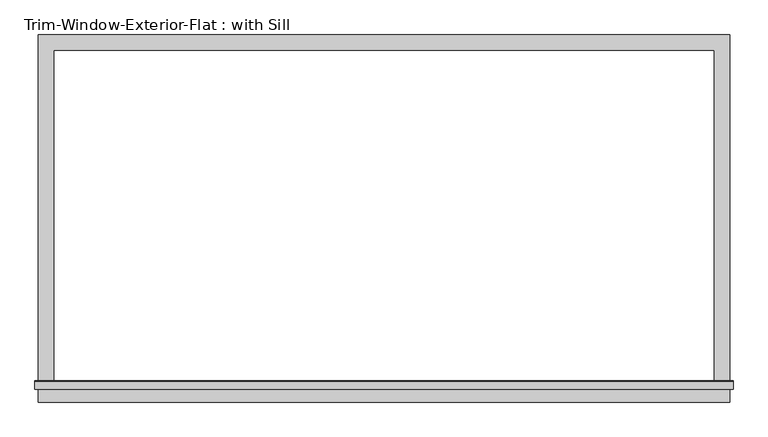
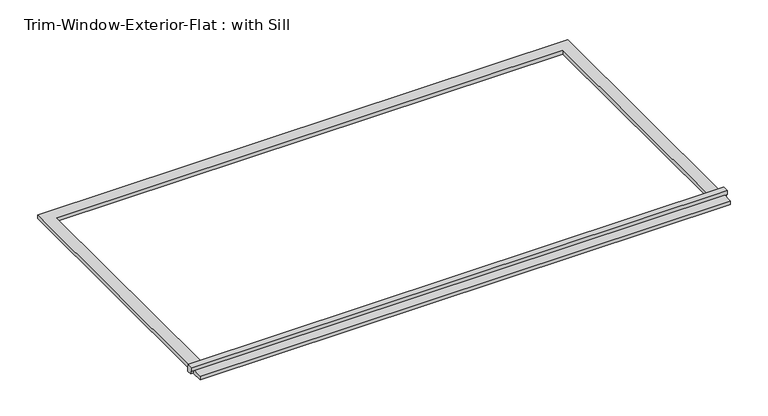
"""IFC4 building model written with IfcOpenShell, lengths in millimetres: proxy geometry, Trim-Window-Exterior-Flat : with Sill."""

from ifc_helpers import new_model, si_unit, frame, origin, origin_with_axes, place, context, project, spatial, polyline, outline, extrude, source, transform, mapped, element, save


def trim_window_exterior_flat_with_sill_4ebd5beb(model_context):
    return source(origin(), model_context, "Body", "SweptSolid", [
        extrude(outline(polyline([(1276.35, -1241.3823709), (1276.35, -1298.5323709), (-1276.35, -1298.5323709), (-1276.35, -1241.3823709), (1276.35, -1241.3823709)])), origin_with_axes(), (0.0, 0.0, 1.0), 19.05),
        extrude(outline(polyline([(-1250.95, 38.1), (-1221.6580645, 38.1), (-1219.2, 19.05), (-1219.2, 0.0), (-1241.3823709, 0.0), (-1241.3823709, 19.05), (-1250.95, 19.05), (-1250.95, 38.1)])), frame((-1289.05, 0.0, 0.0), z_axis=(1.0, 0.0, 0.0), x_axis=(0.0, 1.0, 0.0)), (0.0, 0.0, 1.0), 2578.1),
        extrude(outline(polyline([(-1276.35, 57.15), (1276.35, 57.15), (1276.35, -1219.2), (1219.2, -1219.2), (1219.2, 0.0), (-1219.2, 0.0), (-1219.2, -1219.2), (-1276.35, -1219.2), (-1276.35, 57.15)])), origin_with_axes(), (0.0, 0.0, 1.0), 19.05),
    ])


if __name__ == "__main__":
    model = new_model("IFC4")
    model_context = context("Model", 3, world=origin())
    ifc_project = project(units=[si_unit("LENGTHUNIT", "METRE", prefix="MILLI")], contexts=[model_context])
    site = spatial("IfcSite", under=ifc_project)
    building = spatial("IfcBuilding", under=site)
    placement = place(None, origin())
    trim_window_exterior_flat_with_sill_shape = trim_window_exterior_flat_with_sill_4ebd5beb(model_context)
    element("IfcBuildingElementProxy", 1, Name="Trim-Window-Exterior-Flat : with Sill", ObjectType="Trim-Window-Exterior-Flat : with Sill", at=placement, inside=building, context=model_context, shape_type="MappedRepresentation", body=[
        mapped(trim_window_exterior_flat_with_sill_shape, transform((0.0, 0.0, 0.0), x_axis=(1.0, 0.0, 0.0), y_axis=(0.0, 1.0, 0.0), z_axis=(0.0, 0.0, 1.0))),
    ])
    save(model, "model.ifc")

# Revit data of these elements
# Type "Trim-Window-Exterior-Flat : with Sill"
#   Trim Width = 0' - 2 1/4"
#   Trim Thickness_Picture Frame = 0' - 1 1/4"
#   Trim Thickness_with Sill = 0' - 0 3/4"
#   Sill Thickness = 0' - 1 1/4"
#   Opening Width [instance default] = 2' - 0"
#   Opening Height [instance default] = 3' - 0"
#   Default Elevation = 4' - 0"
#   Sill = yes
#   Picture Frame = no
#   Trim Material [instance default] = none
# Element 1 (IfcBuildingElementProxy, "Trim-Window-Exterior-Flat : with Sill")
#   Opening Width = 8' - 0"
#   Opening Height = 4' - 0"
#   Trim Material = Clad - White
#   Materials on its faces: "Clad - White"
# Materials
#   "Clad - White": class "Wood", colour RGB 242 242 238, transparency 0, Cost = 0
